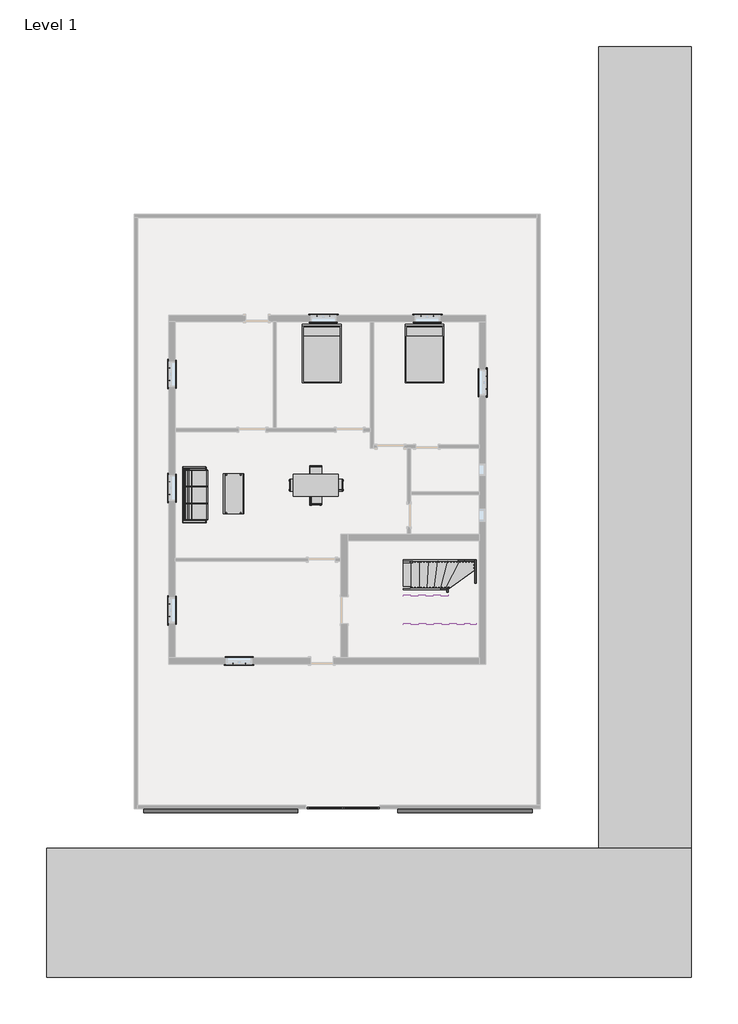
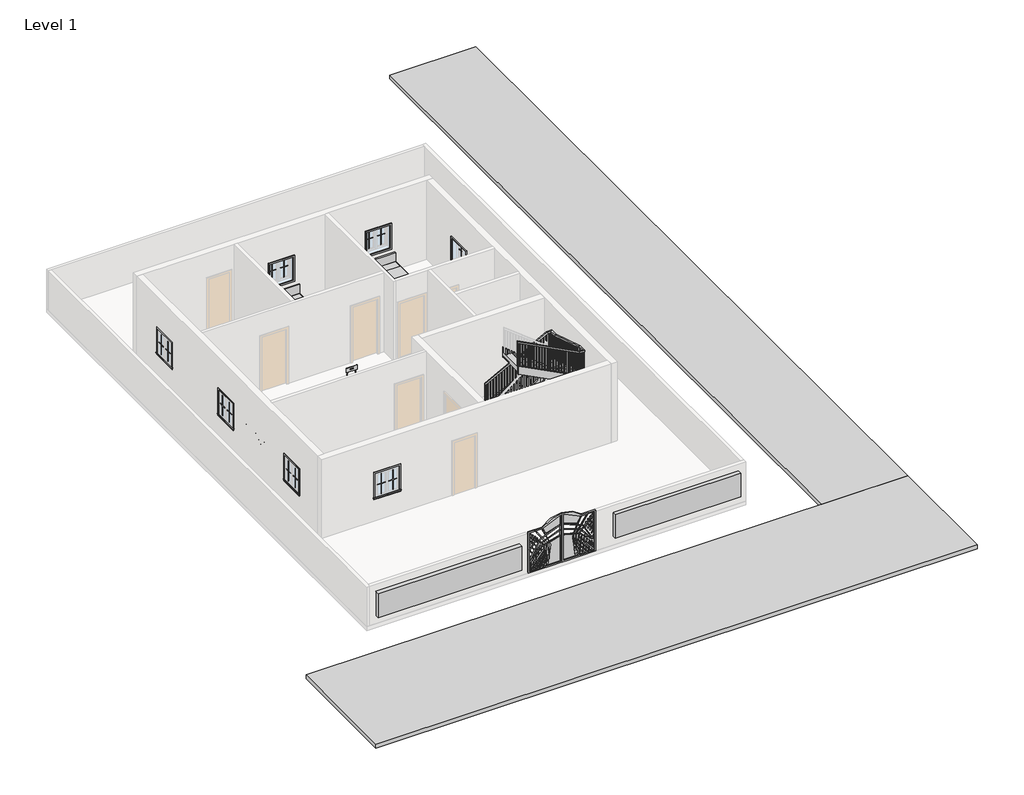
# One storey, part 2 of 2: 33 proxies, 8 members, 4 furniture elements, 1 railing, 1 stair flight.
"""IFC4 building model written with IfcOpenShell, lengths in millimetres."""

from ifc_helpers import new_model, si_unit, frame, origin, place, context, project, spatial, polyline, outline, extrude, faceted_brep, transform, mapped, element, save
from components import generic_models_6bc30956, generic_models_1_generic_models_1_e0ba6133, generic_models_2_generic_models_2_f94be15d, generic_models_3_generic_models_3_0a93b2c0, modern_coffee_table_17989_modern_coffee_table_17989_d3a860c8, muntin_pattern_2x2_muntin_pattern_2x2_b3fe6957, muntin_pattern_2x2_muntin_pattern_2x2_3e0ecaf2, trim_window_exterior_flat_with_sill_41619996, trim_window_interior_flat_picture_frame_51c85655, furniture_2fc85b74, furniture_29a9adb8, furniture_57072a26, bed_17739_bed_17739_15c61121, dining_table_w_chairs_11374_0cdfc61b, stair_flight_a0830a8a

model = new_model("IFC4")

# Units and contexts
model_context = context("Model", 3, world=origin())
ifc_project = project(units=[si_unit("LENGTHUNIT", "METRE", prefix="MILLI")], contexts=[model_context])

# Site, building, storey
site = spatial("IfcSite", under=ifc_project)
building = spatial("IfcBuilding", under=site)
storey = spatial("IfcBuildingStorey", under=building, Name="Level 1", Elevation=0.0)

# Proxies
placement = place(None, origin())
generic_models_shape = generic_models_6bc30956(model_context)
element("IfcBuildingElementProxy", 1, Name="Generic Models", at=placement, inside=storey, context=model_context, shape_type="MappedRepresentation", body=[
    mapped(generic_models_shape, transform((-701.8717864, -9622.1503266, 0.0), x_axis=(1.0, 0.0, 0.0), y_axis=(0.0, 1.0, 0.0), z_axis=(0.0, 0.0, 1.0))),
])
generic_models_1_generic_models_1_shape = generic_models_1_generic_models_1_e0ba6133(model_context)
element("IfcBuildingElementProxy", 2, Name="Generic Models 1 : Generic Models 1", ObjectType="Generic Models 1 : Generic Models 1", at=placement, inside=storey, context=model_context, shape_type="MappedRepresentation", body=[
    mapped(generic_models_1_generic_models_1_shape, transform((0.0, 0.0, 0.0), x_axis=(1.0, 0.0, 0.0), y_axis=(0.0, 1.0, 0.0), z_axis=(0.0, 0.0, 1.0))),
])
generic_models_2_generic_models_2_shape = generic_models_2_generic_models_2_f94be15d(model_context)
element("IfcBuildingElementProxy", 3, Name="Generic Models 2 : Generic Models 2", ObjectType="Generic Models 2 : Generic Models 2", at=placement, inside=storey, context=model_context, shape_type="MappedRepresentation", body=[
    mapped(generic_models_2_generic_models_2_shape, transform((0.0, 0.0, 0.0), x_axis=(1.0, 0.0, 0.0), y_axis=(0.0, 1.0, 0.0), z_axis=(0.0, 0.0, 1.0))),
])
generic_models_3_generic_models_3_shape = generic_models_3_generic_models_3_0a93b2c0(model_context)
element("IfcBuildingElementProxy", 4, Name="Generic Models 3 : Generic Models 3", ObjectType="Generic Models 3 : Generic Models 3", at=placement, inside=storey, context=model_context, shape_type="MappedRepresentation", body=[
    mapped(generic_models_3_generic_models_3_shape, transform((0.0, 0.0, 0.0), x_axis=(1.0, 0.0, 0.0), y_axis=(0.0, 1.0, 0.0), z_axis=(0.0, 0.0, 1.0))),
])
modern_coffee_table_17989_modern_coffee_table_17989_shape = modern_coffee_table_17989_modern_coffee_table_17989_d3a860c8(model_context)
element("IfcBuildingElementProxy", 5, Name="Modern_Coffee_Table_17989 : Modern_Coffee_Table_17989", ObjectType="Modern_Coffee_Table_17989 : Modern_Coffee_Table_17989", at=placement, inside=storey, context=model_context, shape_type="MappedRepresentation", body=[
    mapped(modern_coffee_table_17989_modern_coffee_table_17989_shape, transform((-4791.7841049, 1283.3840961, 0.0), x_axis=(0.0, 1.0, 0.0), y_axis=(-1.0, 0.0, 0.0), z_axis=(0.0, 0.0, 1.0))),
])
muntin_pattern_2x2_muntin_pattern_2x2_shape = muntin_pattern_2x2_muntin_pattern_2x2_b3fe6957(model_context)
element("IfcBuildingElementProxy", 6, Name="Muntin Pattern_2x2 : Muntin Pattern_2x2", ObjectType="Muntin Pattern_2x2 : Muntin Pattern_2x2", at=placement, inside=storey, context=model_context, shape_type="MappedRepresentation", body=[
    mapped(muntin_pattern_2x2_muntin_pattern_2x2_shape, transform((-1586.7442864, 7129.6784997, 984.25), x_axis=(1.0, 0.0, 0.0), y_axis=(0.0, 1.0, 0.0), z_axis=(0.0, 0.0, 1.0))),
])
element("IfcBuildingElementProxy", 7, Name="Muntin Pattern_2x2 : Muntin Pattern_2x2", ObjectType="Muntin Pattern_2x2 : Muntin Pattern_2x2", at=placement, inside=storey, context=model_context, shape_type="MappedRepresentation", body=[
    mapped(muntin_pattern_2x2_muntin_pattern_2x2_shape, transform((1952.1107136, 7129.6784997, 984.25), x_axis=(1.0, 0.0, 0.0), y_axis=(0.0, 1.0, 0.0), z_axis=(0.0, 0.0, 1.0))),
])
element("IfcBuildingElementProxy", 8, Name="Muntin Pattern_2x2 : Muntin Pattern_2x2", ObjectType="Muntin Pattern_2x2 : Muntin Pattern_2x2", at=placement, inside=storey, context=model_context, shape_type="MappedRepresentation", body=[
    mapped(muntin_pattern_2x2_muntin_pattern_2x2_shape, transform((-6633.4067864, 4915.1159997, 984.25), x_axis=(0.0, 1.0, 0.0), y_axis=(-1.0, 0.0, 0.0), z_axis=(0.0, 0.0, 1.0))),
])
element("IfcBuildingElementProxy", 9, Name="Muntin Pattern_2x2 : Muntin Pattern_2x2", ObjectType="Muntin Pattern_2x2 : Muntin Pattern_2x2", at=placement, inside=storey, context=model_context, shape_type="MappedRepresentation", body=[
    mapped(muntin_pattern_2x2_muntin_pattern_2x2_shape, transform((-6633.4067864, 1038.4409997, 984.25), x_axis=(0.0, 1.0, 0.0), y_axis=(-1.0, 0.0, 0.0), z_axis=(0.0, 0.0, 1.0))),
])
element("IfcBuildingElementProxy", 10, Name="Muntin Pattern_2x2 : Muntin Pattern_2x2", ObjectType="Muntin Pattern_2x2 : Muntin Pattern_2x2", at=placement, inside=storey, context=model_context, shape_type="MappedRepresentation", body=[
    mapped(muntin_pattern_2x2_muntin_pattern_2x2_shape, transform((4152.7032136, 5057.9909997, 984.25), x_axis=(0.0, -1.0, 0.0), y_axis=(1.0, 0.0, 0.0), z_axis=(0.0, 0.0, 1.0))),
])
element("IfcBuildingElementProxy", 11, Name="Muntin Pattern_2x2 : Muntin Pattern_2x2", ObjectType="Muntin Pattern_2x2 : Muntin Pattern_2x2", at=placement, inside=storey, context=model_context, shape_type="MappedRepresentation", body=[
    mapped(muntin_pattern_2x2_muntin_pattern_2x2_shape, transform((-6633.4067864, -3125.2540003, 984.25), x_axis=(0.0, 1.0, 0.0), y_axis=(-1.0, 0.0, 0.0), z_axis=(0.0, 0.0, 1.0))),
])
element("IfcBuildingElementProxy", 12, Name="Muntin Pattern_2x2 : Muntin Pattern_2x2", ObjectType="Muntin Pattern_2x2 : Muntin Pattern_2x2", at=placement, inside=storey, context=model_context, shape_type="MappedRepresentation", body=[
    mapped(muntin_pattern_2x2_muntin_pattern_2x2_shape, transform((-4028.3192864, -4738.4715003, 984.25), x_axis=(-1.0, 0.0, 0.0), y_axis=(0.0, -1.0, 0.0), z_axis=(0.0, 0.0, 1.0))),
])
muntin_pattern_2x2_muntin_pattern_2x2_2_shape = muntin_pattern_2x2_muntin_pattern_2x2_3e0ecaf2(model_context)
element("IfcBuildingElementProxy", 13, Name="Muntin Pattern_2x2 : Muntin Pattern_2x2", ObjectType="Muntin Pattern_2x2 : Muntin Pattern_2x2", at=placement, inside=storey, context=model_context, shape_type="MappedRepresentation", body=[
    mapped(muntin_pattern_2x2_muntin_pattern_2x2_2_shape, transform((-1158.1192864, 7129.6784997, 984.25), x_axis=(-1.0, 0.0, 0.0), y_axis=(0.0, -1.0, 0.0), z_axis=(0.0, 0.0, 1.0))),
])
element("IfcBuildingElementProxy", 14, Name="Muntin Pattern_2x2 : Muntin Pattern_2x2", ObjectType="Muntin Pattern_2x2 : Muntin Pattern_2x2", at=placement, inside=storey, context=model_context, shape_type="MappedRepresentation", body=[
    mapped(muntin_pattern_2x2_muntin_pattern_2x2_2_shape, transform((2380.7357136, 7129.6784997, 984.25), x_axis=(-1.0, 0.0, 0.0), y_axis=(0.0, -1.0, 0.0), z_axis=(0.0, 0.0, 1.0))),
])
element("IfcBuildingElementProxy", 15, Name="Muntin Pattern_2x2 : Muntin Pattern_2x2", ObjectType="Muntin Pattern_2x2 : Muntin Pattern_2x2", at=placement, inside=storey, context=model_context, shape_type="MappedRepresentation", body=[
    mapped(muntin_pattern_2x2_muntin_pattern_2x2_2_shape, transform((-6633.4067864, 5343.7409997, 984.25), x_axis=(0.0, -1.0, 0.0), y_axis=(1.0, 0.0, 0.0), z_axis=(0.0, 0.0, 1.0))),
])
element("IfcBuildingElementProxy", 16, Name="Muntin Pattern_2x2 : Muntin Pattern_2x2", ObjectType="Muntin Pattern_2x2 : Muntin Pattern_2x2", at=placement, inside=storey, context=model_context, shape_type="MappedRepresentation", body=[
    mapped(muntin_pattern_2x2_muntin_pattern_2x2_2_shape, transform((-6633.4067864, 1467.0659997, 984.25), x_axis=(0.0, -1.0, 0.0), y_axis=(1.0, 0.0, 0.0), z_axis=(0.0, 0.0, 1.0))),
])
element("IfcBuildingElementProxy", 17, Name="Muntin Pattern_2x2 : Muntin Pattern_2x2", ObjectType="Muntin Pattern_2x2 : Muntin Pattern_2x2", at=placement, inside=storey, context=model_context, shape_type="MappedRepresentation", body=[
    mapped(muntin_pattern_2x2_muntin_pattern_2x2_2_shape, transform((4152.7032136, 4629.3659997, 984.25), x_axis=(0.0, 1.0, 0.0), y_axis=(-1.0, 0.0, 0.0), z_axis=(0.0, 0.0, 1.0))),
])
element("IfcBuildingElementProxy", 18, Name="Muntin Pattern_2x2 : Muntin Pattern_2x2", ObjectType="Muntin Pattern_2x2 : Muntin Pattern_2x2", at=placement, inside=storey, context=model_context, shape_type="MappedRepresentation", body=[
    mapped(muntin_pattern_2x2_muntin_pattern_2x2_2_shape, transform((-6633.4067864, -2696.6290003, 984.25), x_axis=(0.0, -1.0, 0.0), y_axis=(1.0, 0.0, 0.0), z_axis=(0.0, 0.0, 1.0))),
])
element("IfcBuildingElementProxy", 19, Name="Muntin Pattern_2x2 : Muntin Pattern_2x2", ObjectType="Muntin Pattern_2x2 : Muntin Pattern_2x2", at=placement, inside=storey, context=model_context, shape_type="MappedRepresentation", body=[
    mapped(muntin_pattern_2x2_muntin_pattern_2x2_2_shape, transform((-4456.9442864, -4738.4715003, 984.25), x_axis=(1.0, 0.0, 0.0), y_axis=(0.0, 1.0, 0.0), z_axis=(0.0, 0.0, 1.0))),
])
trim_window_exterior_flat_with_sill_shape = trim_window_exterior_flat_with_sill_41619996(model_context)
element("IfcBuildingElementProxy", 20, Name="Trim-Window-Exterior-Flat : with Sill", ObjectType="Trim-Window-Exterior-Flat : with Sill", at=placement, inside=storey, context=model_context, shape_type="MappedRepresentation", body=[
    mapped(trim_window_exterior_flat_with_sill_shape, transform((-1372.4317864, 7139.2034997, 1828.8), x_axis=(-1.0, 0.0, 0.0), y_axis=(0.0, 0.0, 1.0), z_axis=(0.0, 1.0, 0.0))),
])
element("IfcBuildingElementProxy", 21, Name="Trim-Window-Exterior-Flat : with Sill", ObjectType="Trim-Window-Exterior-Flat : with Sill", at=placement, inside=storey, context=model_context, shape_type="MappedRepresentation", body=[
    mapped(trim_window_exterior_flat_with_sill_shape, transform((2166.4232136, 7139.2034997, 1828.8), x_axis=(-1.0, 0.0, 0.0), y_axis=(0.0, 0.0, 1.0), z_axis=(0.0, 1.0, 0.0))),
])
element("IfcBuildingElementProxy", 22, Name="Trim-Window-Exterior-Flat : with Sill", ObjectType="Trim-Window-Exterior-Flat : with Sill", at=placement, inside=storey, context=model_context, shape_type="MappedRepresentation", body=[
    mapped(trim_window_exterior_flat_with_sill_shape, transform((-6642.9317864, 5129.4284997, 1828.8), x_axis=(0.0, -1.0, 0.0), y_axis=(0.0, 0.0, 1.0), z_axis=(-1.0, 0.0, 0.0))),
])
element("IfcBuildingElementProxy", 23, Name="Trim-Window-Exterior-Flat : with Sill", ObjectType="Trim-Window-Exterior-Flat : with Sill", at=placement, inside=storey, context=model_context, shape_type="MappedRepresentation", body=[
    mapped(trim_window_exterior_flat_with_sill_shape, transform((-6642.9317864, 1252.7534997, 1828.8), x_axis=(0.0, -1.0, 0.0), y_axis=(0.0, 0.0, 1.0), z_axis=(-1.0, 0.0, 0.0))),
])
element("IfcBuildingElementProxy", 24, Name="Trim-Window-Exterior-Flat : with Sill", ObjectType="Trim-Window-Exterior-Flat : with Sill", at=placement, inside=storey, context=model_context, shape_type="MappedRepresentation", body=[
    mapped(trim_window_exterior_flat_with_sill_shape, transform((4162.2282136, 4843.6784997, 1828.8), x_axis=(0.0, 1.0, 0.0), y_axis=(0.0, 0.0, 1.0), z_axis=(1.0, 0.0, 0.0))),
])
element("IfcBuildingElementProxy", 25, Name="Trim-Window-Exterior-Flat : with Sill", ObjectType="Trim-Window-Exterior-Flat : with Sill", at=placement, inside=storey, context=model_context, shape_type="MappedRepresentation", body=[
    mapped(trim_window_exterior_flat_with_sill_shape, transform((-6642.9317864, -2910.9415003, 1828.8), x_axis=(0.0, -1.0, 0.0), y_axis=(0.0, 0.0, 1.0), z_axis=(-1.0, 0.0, 0.0))),
])
element("IfcBuildingElementProxy", 26, Name="Trim-Window-Exterior-Flat : with Sill", ObjectType="Trim-Window-Exterior-Flat : with Sill", at=placement, inside=storey, context=model_context, shape_type="MappedRepresentation", body=[
    mapped(trim_window_exterior_flat_with_sill_shape, transform((-4242.6317864, -4747.9965003, 1828.8), x_axis=(1.0, 0.0, 0.0), y_axis=(0.0, 0.0, 1.0), z_axis=(0.0, -1.0, 0.0))),
])
trim_window_interior_flat_picture_frame_shape = trim_window_interior_flat_picture_frame_51c85655(model_context)
element("IfcBuildingElementProxy", 27, Name="Trim-Window-Interior-Flat : Picture Frame", ObjectType="Trim-Window-Interior-Flat : Picture Frame", at=placement, inside=storey, context=model_context, shape_type="MappedRepresentation", body=[
    mapped(trim_window_interior_flat_picture_frame_shape, transform((-1372.4317864, 6910.6034997, 1828.8), x_axis=(1.0, 0.0, 0.0), y_axis=(0.0, 0.0, 1.0), z_axis=(0.0, -1.0, 0.0))),
])
element("IfcBuildingElementProxy", 28, Name="Trim-Window-Interior-Flat : Picture Frame", ObjectType="Trim-Window-Interior-Flat : Picture Frame", at=placement, inside=storey, context=model_context, shape_type="MappedRepresentation", body=[
    mapped(trim_window_interior_flat_picture_frame_shape, transform((2166.4232136, 6910.6034997, 1828.8), x_axis=(1.0, 0.0, 0.0), y_axis=(0.0, 0.0, 1.0), z_axis=(0.0, -1.0, 0.0))),
])
element("IfcBuildingElementProxy", 29, Name="Trim-Window-Interior-Flat : Picture Frame", ObjectType="Trim-Window-Interior-Flat : Picture Frame", at=placement, inside=storey, context=model_context, shape_type="MappedRepresentation", body=[
    mapped(trim_window_interior_flat_picture_frame_shape, transform((-6414.3317864, 5129.4284997, 1828.8), x_axis=(0.0, 1.0, 0.0), y_axis=(0.0, 0.0, 1.0), z_axis=(1.0, 0.0, 0.0))),
])
element("IfcBuildingElementProxy", 30, Name="Trim-Window-Interior-Flat : Picture Frame", ObjectType="Trim-Window-Interior-Flat : Picture Frame", at=placement, inside=storey, context=model_context, shape_type="MappedRepresentation", body=[
    mapped(trim_window_interior_flat_picture_frame_shape, transform((-6414.3317864, 1252.7534997, 1828.8), x_axis=(0.0, 1.0, 0.0), y_axis=(0.0, 0.0, 1.0), z_axis=(1.0, 0.0, 0.0))),
])
element("IfcBuildingElementProxy", 31, Name="Trim-Window-Interior-Flat : Picture Frame", ObjectType="Trim-Window-Interior-Flat : Picture Frame", at=placement, inside=storey, context=model_context, shape_type="MappedRepresentation", body=[
    mapped(trim_window_interior_flat_picture_frame_shape, transform((3933.6282136, 4843.6784997, 1828.8), x_axis=(0.0, -1.0, 0.0), y_axis=(0.0, 0.0, 1.0), z_axis=(-1.0, 0.0, 0.0))),
])
element("IfcBuildingElementProxy", 32, Name="Trim-Window-Interior-Flat : Picture Frame", ObjectType="Trim-Window-Interior-Flat : Picture Frame", at=placement, inside=storey, context=model_context, shape_type="MappedRepresentation", body=[
    mapped(trim_window_interior_flat_picture_frame_shape, transform((-6414.3317864, -2910.9415003, 1828.8), x_axis=(0.0, 1.0, 0.0), y_axis=(0.0, 0.0, 1.0), z_axis=(1.0, 0.0, 0.0))),
])
element("IfcBuildingElementProxy", 33, Name="Trim-Window-Interior-Flat : Picture Frame", ObjectType="Trim-Window-Interior-Flat : Picture Frame", at=placement, inside=storey, context=model_context, shape_type="MappedRepresentation", body=[
    mapped(trim_window_interior_flat_picture_frame_shape, transform((-4242.6317864, -4519.3965003, 1828.8), x_axis=(-1.0, 0.0, 0.0), y_axis=(0.0, 0.0, 1.0), z_axis=(0.0, 1.0, 0.0))),
])

# Furniture
furniture_shape = furniture_2fc85b74(model_context)
furniture_2_shape = furniture_29a9adb8(model_context)
furniture_3_shape = furniture_57072a26(model_context)
element("IfcFurniture", 34, at=placement, inside=storey, context=model_context, shape_type="MappedRepresentation", body=[
    mapped(furniture_shape, transform((-5371.0104604, 1017.8034997, 0.0), x_axis=(0.0, 1.0, 0.0), y_axis=(-1.0, 0.0, 0.0), z_axis=(0.0, 0.0, 1.0))),
    mapped(furniture_2_shape, transform((-5371.0104604, 1017.8034997, 0.0), x_axis=(0.0, 1.0, 0.0), y_axis=(-1.0, 0.0, 0.0), z_axis=(0.0, 0.0, 1.0))),
    mapped(furniture_3_shape, transform((-5371.0104604, 1017.8034997, 0.0), x_axis=(0.0, 1.0, 0.0), y_axis=(-1.0, 0.0, 0.0), z_axis=(0.0, 0.0, 1.0))),
])
bed_17739_bed_17739_shape = bed_17739_bed_17739_15c61121(model_context)
element("IfcFurniture", 35, ObjectType="Bed_17739 : Bed_17739", at=placement, inside=storey, context=model_context, shape_type="MappedRepresentation", body=[
    mapped(bed_17739_bed_17739_shape, transform((-1425.7717864, 5805.7034997, 0.0), x_axis=(1.0, 0.0, 0.0), y_axis=(0.0, 1.0, 0.0), z_axis=(0.0, 0.0, 1.0))),
])
element("IfcFurniture", 36, ObjectType="Bed_17739 : Bed_17739", at=placement, inside=storey, context=model_context, shape_type="MappedRepresentation", body=[
    mapped(bed_17739_bed_17739_shape, transform((2066.7282136, 5805.7034997, 0.0), x_axis=(1.0, 0.0, 0.0), y_axis=(0.0, 1.0, 0.0), z_axis=(0.0, 0.0, 1.0))),
])
dining_table_w_chairs_11374_shape = dining_table_w_chairs_11374_0cdfc61b(model_context)
element("IfcFurniture", 37, ObjectType="Dining_Table_w_Chairs_11374", at=placement, inside=storey, context=model_context, shape_type="MappedRepresentation", body=[
    mapped(dining_table_w_chairs_11374_shape, transform((-1657.0397106, 1252.0888157, 0.0), x_axis=(1.0, 0.0, 0.0), y_axis=(0.0, 1.0, 0.0), z_axis=(0.0, 0.0, 1.0))),
])

# Members
element("IfcMember", 38, ObjectType="Stringer - 2\" Width", at=placement, inside=storey, context=model_context, shape_type="SweptSolid", body=[
    extrude(outline(polyline([(229.639954, 1342.8282136), (0.0, 1342.8282136), (0.0, 1562.5905312), (962.500629, 3430.2454053), (1305.3956453, 3430.2454053), (229.639954, 1342.8282136)])), frame((0.0, -1245.3365003, 0.0), z_axis=(0.0, 1.0, 0.0), x_axis=(0.0, 0.0, 1.0)), (0.0, 0.0, 1.0), 50.8),
])
element("IfcMember", 39, ObjectType="Stringer - 2\" Width", at=placement, inside=storey, context=model_context, shape_type="SweptSolid", body=[
    extrude(outline(polyline([(3430.2454053, -1245.3365003), (3430.2454053, -1194.5365003), (3784.9599055, -1194.5365003), (3784.9599055, -1245.3365003), (3430.2454053, -1245.3365003)])), frame((0.0, 0.0, 962.500629), z_axis=(0.0, 0.0, 1.0), x_axis=(1.0, 0.0, 0.0)), (0.0, 0.0, 1.0), 342.8950162),
])
element("IfcMember", 40, ObjectType="Stringer - 2\" Width", at=placement, inside=storey, context=model_context, shape_type="SweptSolid", body=[
    extrude(outline(polyline([(-1194.5365003, 1289.0952212), (-1194.5365003, 1000.5956453), (-1364.0589833, 1000.5956453), (-3353.5365003, 1638.9682298), (-3353.5365003, 1969.9972697), (-3316.5563831, 1969.9972697), (-1194.5365003, 1289.0952212)])), frame((3784.9599055, 0.0, 0.0), z_axis=(1.0, 0.0, 0.0), x_axis=(0.0, 1.0, 0.0)), (0.0, 0.0, 1.0), 50.8),
])
element("IfcMember", 41, ObjectType="Stringer - 2\" Width", at=placement, inside=storey, context=model_context, shape_type="SweptSolid", body=[
    extrude(outline(polyline([(3835.7599055, -3353.5365003), (3835.7599055, -3404.3365003), (3430.2454053, -3404.3365003), (3430.2454053, -3353.5365003), (3835.7599055, -3353.5365003)])), frame((0.0, 0.0, 1649.8904473), z_axis=(0.0, 0.0, 1.0), x_axis=(1.0, 0.0, 0.0)), (0.0, 0.0, 1.0), 320.1068224),
])
element("IfcMember", 42, ObjectType="Stringer - 2\" Width", at=placement, inside=storey, context=model_context, shape_type="SweptSolid", body=[
    extrude(outline(polyline([(1649.8904473, 3430.2454053), (1969.9972697, 3430.2454053), (3045.7529609, 1342.8282136), (2725.6461385, 1342.8282136), (1649.8904473, 3430.2454053)])), frame((0.0, -3404.3365003, 0.0), z_axis=(0.0, 1.0, 0.0), x_axis=(0.0, 0.0, 1.0)), (0.0, 0.0, 1.0), 50.8),
])
element("IfcMember", 43, ObjectType="Stringer - 2\" Width", at=placement, inside=storey, context=model_context, shape_type="SweptSolid", body=[
    extrude(outline(polyline([(176.1764461, 1342.8282136), (0.0, 1342.8282136), (0.0, 1609.0898582), (987.1410923, 2819.7599055), (1380.418648, 2819.7599055), (176.1764461, 1342.8282136)])), frame((0.0, -2210.5365003, 0.0), z_axis=(0.0, 1.0, 0.0), x_axis=(0.0, 0.0, 1.0)), (0.0, 0.0, 1.0), 50.8),
])
element("IfcMember", 44, ObjectType="Stringer - 2\" Width", at=placement, inside=storey, context=model_context, shape_type="SweptSolid", body=[
    extrude(outline(polyline([(-2159.7365003, 1573.2682978), (-2159.7365003, 1028.5617647), (-2193.9787177, 1028.5617647), (-2388.3365003, 1360.465107), (-2388.3365003, 1926.1409689), (-2366.3736178, 1926.1409689), (-2159.7365003, 1573.2682978)])), frame((2819.7599055, 0.0, 0.0), z_axis=(1.0, 0.0, 0.0), x_axis=(0.0, 1.0, 0.0)), (0.0, 0.0, 1.0), 50.8),
])
element("IfcMember", 45, ObjectType="Stringer - 2\" Width", at=placement, inside=storey, context=model_context, shape_type="SweptSolid", body=[
    extrude(outline(polyline([(1532.8634131, 2870.5599055), (1926.1409689, 2870.5599055), (3171.8038432, 1342.8282136), (2778.5262875, 1342.8282136), (1532.8634131, 2870.5599055)])), frame((0.0, -2439.1365003, 0.0), z_axis=(0.0, 1.0, 0.0), x_axis=(0.0, 0.0, 1.0)), (0.0, 0.0, 1.0), 50.8),
])

# Railing
element("IfcRailing", 46, ObjectType="Handrail - Rectangular", at=placement, inside=storey, context=model_context, shape_type="SolidModel", body=[
    faceted_brep([(1342.8282136, -1245.3365003, 1083.7333333), (1342.8282136, -1245.3365003, 1026.2742652), (1342.8282136, -1296.1365003, 1026.2742652), (1342.8282136, -1296.1365003, 1083.7333333), (3600.5532757, -1245.3365003, 2277.0239201), (3613.1523402, -1245.3365003, 2226.2239201), (3613.1523402, -1296.1365003, 2226.2239201), (3600.5532757, -1296.1365003, 2277.0239201), (3784.9599055, -1245.3365003, 2277.0239201), (3784.9599055, -1245.3365003, 2226.2239201), (3734.1599055, -1296.1365003, 2226.2239201), (3734.1599055, -1296.1365003, 2277.0239201), (3784.9599055, -1532.6483825, 2277.0239201), (3784.9599055, -1540.5989586, 2226.2239201), (3734.1599055, -1540.5989586, 2226.2239201), (3734.1599055, -1532.6483825, 2277.0239201), (3784.9599055, -3066.2246182, 2769.1094132), (3784.9599055, -3074.1751943, 2718.3094132), (3734.1599055, -3074.1751943, 2718.3094132), (3734.1599055, -3066.2246182, 2769.1094132), (3784.9599055, -3353.5365003, 2769.1094132), (3784.9599055, -3353.5365003, 2718.3094132), (3734.1599055, -3302.7365003, 2718.3094132), (3734.1599055, -3302.7365003, 2769.1094132), (3600.5532757, -3353.5365003, 2769.1094132), (3587.9542112, -3353.5365003, 2718.3094132), (3587.9542112, -3302.7365003, 2718.3094132), (3600.5532757, -3302.7365003, 2769.1094132), (1342.8282136, -3353.5365003, 3962.4), (1342.8282136, -3302.7365003, 3962.4), (1342.8282136, -3302.7365003, 3904.9409318), (1342.8282136, -3353.5365003, 3904.9409318)], [[[0, 1, 2, 3]], [[1, 0, 4, 5]], [[2, 1, 5, 6]], [[3, 2, 6, 7]], [[0, 3, 7, 4]], [[5, 4, 8, 9]], [[6, 5, 9, 10]], [[7, 6, 10, 11]], [[4, 7, 11, 8]], [[9, 8, 12, 13]], [[10, 9, 13, 14]], [[11, 10, 14, 15]], [[8, 11, 15, 12]], [[13, 12, 16, 17]], [[14, 13, 17, 18]], [[15, 14, 18, 19]], [[12, 15, 19, 16]], [[17, 16, 20, 21]], [[18, 17, 21, 22]], [[19, 18, 22, 23]], [[16, 19, 23, 20]], [[21, 20, 24, 25]], [[22, 21, 25, 26]], [[23, 22, 26, 27]], [[20, 23, 27, 24]], [[28, 29, 30, 31]], [[25, 24, 28, 31]], [[26, 25, 31, 30]], [[27, 26, 30, 29]], [[24, 27, 29, 28]]]),
    extrude(outline(polyline([(3867.7284102, 1413.2349055), (2878.6666667, 1413.2349055), (2878.6666667, 1432.2849055), (3857.6597858, 1432.2849055), (3867.7284102, 1413.2349055)])), frame((0.0, -3337.6615003, 0.0), z_axis=(0.0, 1.0, 0.0), x_axis=(0.0, 0.0, 1.0)), (0.0, 0.0, 1.0), 19.05),
    extrude(outline(polyline([(3814.02908, 1514.8349055), (2878.6666667, 1514.8349055), (2878.6666667, 1533.8849055), (3803.9604556, 1533.8849055), (3814.02908, 1514.8349055)])), frame((0.0, -3337.6615003, 0.0), z_axis=(0.0, 1.0, 0.0), x_axis=(0.0, 0.0, 1.0)), (0.0, 0.0, 1.0), 19.05),
    extrude(outline(polyline([(3760.3297498, 1616.4349055), (2709.3333333, 1616.4349055), (2709.3333333, 1635.4849055), (3750.2611254, 1635.4849055), (3760.3297498, 1616.4349055)])), frame((0.0, -3337.6615003, 0.0), z_axis=(0.0, 1.0, 0.0), x_axis=(0.0, 0.0, 1.0)), (0.0, 0.0, 1.0), 19.05),
    extrude(outline(polyline([(3706.6304196, 1718.0349055), (2709.3333333, 1718.0349055), (2709.3333333, 1737.0849055), (3696.5617952, 1737.0849055), (3706.6304196, 1718.0349055)])), frame((0.0, -3337.6615003, 0.0), z_axis=(0.0, 1.0, 0.0), x_axis=(0.0, 0.0, 1.0)), (0.0, 0.0, 1.0), 19.05),
    extrude(outline(polyline([(3652.9310894, 1819.6349055), (2709.3333333, 1819.6349055), (2709.3333333, 1838.6849055), (3642.862465, 1838.6849055), (3652.9310894, 1819.6349055)])), frame((0.0, -3337.6615003, 0.0), z_axis=(0.0, 1.0, 0.0), x_axis=(0.0, 0.0, 1.0)), (0.0, 0.0, 1.0), 19.05),
    extrude(outline(polyline([(3599.2317592, 1921.2349055), (2540.0, 1921.2349055), (2540.0, 1940.2849055), (3589.1631348, 1940.2849055), (3599.2317592, 1921.2349055)])), frame((0.0, -3337.6615003, 0.0), z_axis=(0.0, 1.0, 0.0), x_axis=(0.0, 0.0, 1.0)), (0.0, 0.0, 1.0), 19.05),
    extrude(outline(polyline([(3545.532429, 2022.8349055), (2540.0, 2022.8349055), (2540.0, 2041.8849055), (3535.4638046, 2041.8849055), (3545.532429, 2022.8349055)])), frame((0.0, -3337.6615003, 0.0), z_axis=(0.0, 1.0, 0.0), x_axis=(0.0, 0.0, 1.0)), (0.0, 0.0, 1.0), 19.05),
    extrude(outline(polyline([(3491.8330988, 2124.4349055), (2540.0, 2124.4349055), (2540.0, 2143.4849055), (3481.7644744, 2143.4849055), (3491.8330988, 2124.4349055)])), frame((0.0, -3337.6615003, 0.0), z_axis=(0.0, 1.0, 0.0), x_axis=(0.0, 0.0, 1.0)), (0.0, 0.0, 1.0), 19.05),
    extrude(outline(polyline([(3438.1337686, 2226.0349055), (2370.6666667, 2226.0349055), (2370.6666667, 2245.0849055), (3428.0651442, 2245.0849055), (3438.1337686, 2226.0349055)])), frame((0.0, -3337.6615003, 0.0), z_axis=(0.0, 1.0, 0.0), x_axis=(0.0, 0.0, 1.0)), (0.0, 0.0, 1.0), 19.05),
    extrude(outline(polyline([(3384.4344384, 2327.6349055), (2370.6666667, 2327.6349055), (2370.6666667, 2346.6849055), (3374.365814, 2346.6849055), (3384.4344384, 2327.6349055)])), frame((0.0, -3337.6615003, 0.0), z_axis=(0.0, 1.0, 0.0), x_axis=(0.0, 0.0, 1.0)), (0.0, 0.0, 1.0), 19.05),
    extrude(outline(polyline([(3330.7351082, 2429.2349055), (2370.6666667, 2429.2349055), (2370.6666667, 2448.2849055), (3320.6664838, 2448.2849055), (3330.7351082, 2429.2349055)])), frame((0.0, -3337.6615003, 0.0), z_axis=(0.0, 1.0, 0.0), x_axis=(0.0, 0.0, 1.0)), (0.0, 0.0, 1.0), 19.05),
    extrude(outline(polyline([(3277.035778, 2530.8349055), (2201.3333333, 2530.8349055), (2201.3333333, 2549.8849055), (3266.9671536, 2549.8849055), (3277.035778, 2530.8349055)])), frame((0.0, -3337.6615003, 0.0), z_axis=(0.0, 1.0, 0.0), x_axis=(0.0, 0.0, 1.0)), (0.0, 0.0, 1.0), 19.05),
    extrude(outline(polyline([(3223.3364478, 2632.4349055), (2201.3333333, 2632.4349055), (2201.3333333, 2651.4849055), (3213.2678234, 2651.4849055), (3223.3364478, 2632.4349055)])), frame((0.0, -3337.6615003, 0.0), z_axis=(0.0, 1.0, 0.0), x_axis=(0.0, 0.0, 1.0)), (0.0, 0.0, 1.0), 19.05),
    extrude(outline(polyline([(3169.6371176, 2734.0349055), (2201.3333333, 2734.0349055), (2201.3333333, 2753.0849055), (3159.5684932, 2753.0849055), (3169.6371176, 2734.0349055)])), frame((0.0, -3337.6615003, 0.0), z_axis=(0.0, 1.0, 0.0), x_axis=(0.0, 0.0, 1.0)), (0.0, 0.0, 1.0), 19.05),
    extrude(outline(polyline([(3115.9377874, 2835.6349055), (2201.3333333, 2835.6349055), (2201.3333333, 2854.6849055), (3105.869163, 2854.6849055), (3115.9377874, 2835.6349055)])), frame((0.0, -3337.6615003, 0.0), z_axis=(0.0, 1.0, 0.0), x_axis=(0.0, 0.0, 1.0)), (0.0, 0.0, 1.0), 19.05),
    extrude(outline(polyline([(3062.2384572, 2937.2349055), (2032.0, 2937.2349055), (2032.0, 2956.2849055), (3052.1698328, 2956.2849055), (3062.2384572, 2937.2349055)])), frame((0.0, -3337.6615003, 0.0), z_axis=(0.0, 1.0, 0.0), x_axis=(0.0, 0.0, 1.0)), (0.0, 0.0, 1.0), 19.05),
    extrude(outline(polyline([(3008.539127, 3038.8349055), (2032.0, 3038.8349055), (2032.0, 3057.8849055), (2998.4705026, 3057.8849055), (3008.539127, 3038.8349055)])), frame((0.0, -3337.6615003, 0.0), z_axis=(0.0, 1.0, 0.0), x_axis=(0.0, 0.0, 1.0)), (0.0, 0.0, 1.0), 19.05),
    extrude(outline(polyline([(2954.8397968, 3140.4349055), (2032.0, 3140.4349055), (2032.0, 3159.4849055), (2944.7711724, 3159.4849055), (2954.8397968, 3140.4349055)])), frame((0.0, -3337.6615003, 0.0), z_axis=(0.0, 1.0, 0.0), x_axis=(0.0, 0.0, 1.0)), (0.0, 0.0, 1.0), 19.05),
    extrude(outline(polyline([(2901.1404666, 3242.0349055), (2032.0, 3242.0349055), (2032.0, 3261.0849055), (2891.0718422, 3261.0849055), (2901.1404666, 3242.0349055)])), frame((0.0, -3337.6615003, 0.0), z_axis=(0.0, 1.0, 0.0), x_axis=(0.0, 0.0, 1.0)), (0.0, 0.0, 1.0), 19.05),
    extrude(outline(polyline([(2847.4411364, 3343.6349055), (1862.6666667, 3343.6349055), (1862.6666667, 3362.6849055), (2837.372512, 3362.6849055), (2847.4411364, 3343.6349055)])), frame((0.0, -3337.6615003, 0.0), z_axis=(0.0, 1.0, 0.0), x_axis=(0.0, 0.0, 1.0)), (0.0, 0.0, 1.0), 19.05),
    extrude(outline(polyline([(2793.7418062, 3445.2349055), (1862.6666667, 3445.2349055), (1862.6666667, 3464.2849055), (2783.6731818, 3464.2849055), (2793.7418062, 3445.2349055)])), frame((0.0, -3337.6615003, 0.0), z_axis=(0.0, 1.0, 0.0), x_axis=(0.0, 0.0, 1.0)), (0.0, 0.0, 1.0), 19.05),
    extrude(outline(polyline([(2740.042476, 3546.8349055), (1862.6666667, 3546.8349055), (1862.6666667, 3565.8849055), (2729.9738516, 3565.8849055), (2740.042476, 3546.8349055)])), frame((0.0, -3337.6615003, 0.0), z_axis=(0.0, 1.0, 0.0), x_axis=(0.0, 0.0, 1.0)), (0.0, 0.0, 1.0), 19.05),
    extrude(outline(polyline([(3667.4849055, -3337.6615003), (3648.4349055, -3337.6615003), (3648.4349055, -3318.6115003), (3667.4849055, -3318.6115003), (3667.4849055, -3337.6615003)])), frame((0.0, 0.0, 1862.6666667), z_axis=(0.0, 0.0, 1.0), x_axis=(1.0, 0.0, 0.0)), (0.0, 0.0, 1.0), 855.6427466),
    extrude(outline(polyline([(3769.0849055, -3293.2115003), (3769.0849055, -3312.2615003), (3750.0349055, -3312.2615003), (3750.0349055, -3293.2115003), (3769.0849055, -3293.2115003)])), frame((0.0, 0.0, 1862.6666667), z_axis=(0.0, 0.0, 1.0), x_axis=(1.0, 0.0, 0.0)), (0.0, 0.0, 1.0), 855.6427466),
    extrude(outline(polyline([(3769.0849055, -3191.6115003), (3769.0849055, -3210.6615003), (3750.0349055, -3210.6615003), (3750.0349055, -3191.6115003), (3769.0849055, -3191.6115003)])), frame((0.0, 0.0, 1862.6666667), z_axis=(0.0, 0.0, 1.0), x_axis=(1.0, 0.0, 0.0)), (0.0, 0.0, 1.0), 855.6427466),
    extrude(outline(polyline([(3769.0849055, -3090.0115003), (3769.0849055, -3109.0615003), (3750.0349055, -3109.0615003), (3750.0349055, -3090.0115003), (3769.0849055, -3090.0115003)])), frame((0.0, 0.0, 1862.6666667), z_axis=(0.0, 0.0, 1.0), x_axis=(1.0, 0.0, 0.0)), (0.0, 0.0, 1.0), 855.6427466),
    extrude(outline(polyline([(-2988.4115003, 2690.7900316), (-2988.4115003, 1693.3333333), (-3007.4615003, 1693.3333333), (-3007.4615003, 2696.9026907), (-2988.4115003, 2690.7900316)])), frame((3750.0349055, 0.0, 0.0), z_axis=(1.0, 0.0, 0.0), x_axis=(0.0, 1.0, 0.0)), (0.0, 0.0, 1.0), 19.05),
    extrude(outline(polyline([(-2886.8115003, 2658.1891834), (-2886.8115003, 1693.3333333), (-2905.8615003, 1693.3333333), (-2905.8615003, 2664.3018425), (-2886.8115003, 2658.1891834)])), frame((3750.0349055, 0.0, 0.0), z_axis=(1.0, 0.0, 0.0), x_axis=(0.0, 1.0, 0.0)), (0.0, 0.0, 1.0), 19.05),
    extrude(outline(polyline([(-2785.2115003, 2625.5883352), (-2785.2115003, 1693.3333333), (-2804.2615003, 1693.3333333), (-2804.2615003, 2631.7009942), (-2785.2115003, 2625.5883352)])), frame((3750.0349055, 0.0, 0.0), z_axis=(1.0, 0.0, 0.0), x_axis=(0.0, 1.0, 0.0)), (0.0, 0.0, 1.0), 19.05),
    extrude(outline(polyline([(-2683.6115003, 2592.987487), (-2683.6115003, 1693.3333333), (-2702.6615003, 1693.3333333), (-2702.6615003, 2599.100146), (-2683.6115003, 2592.987487)])), frame((3750.0349055, 0.0, 0.0), z_axis=(1.0, 0.0, 0.0), x_axis=(0.0, 1.0, 0.0)), (0.0, 0.0, 1.0), 19.05),
    extrude(outline(polyline([(-2582.0115003, 2560.3866387), (-2582.0115003, 1693.3333333), (-2601.0615003, 1693.3333333), (-2601.0615003, 2566.4992978), (-2582.0115003, 2560.3866387)])), frame((3750.0349055, 0.0, 0.0), z_axis=(1.0, 0.0, 0.0), x_axis=(0.0, 1.0, 0.0)), (0.0, 0.0, 1.0), 19.05),
    extrude(outline(polyline([(-2480.4115003, 2527.7857905), (-2480.4115003, 1524.0), (-2499.4615003, 1524.0), (-2499.4615003, 2533.8984495), (-2480.4115003, 2527.7857905)])), frame((3750.0349055, 0.0, 0.0), z_axis=(1.0, 0.0, 0.0), x_axis=(0.0, 1.0, 0.0)), (0.0, 0.0, 1.0), 19.05),
    extrude(outline(polyline([(-2378.8115003, 2495.1849423), (-2378.8115003, 1524.0), (-2397.8615003, 1524.0), (-2397.8615003, 2501.2976013), (-2378.8115003, 2495.1849423)])), frame((3750.0349055, 0.0, 0.0), z_axis=(1.0, 0.0, 0.0), x_axis=(0.0, 1.0, 0.0)), (0.0, 0.0, 1.0), 19.05),
    extrude(outline(polyline([(-2277.2115003, 2462.5840941), (-2277.2115003, 1524.0), (-2296.2615003, 1524.0), (-2296.2615003, 2468.6967531), (-2277.2115003, 2462.5840941)])), frame((3750.0349055, 0.0, 0.0), z_axis=(1.0, 0.0, 0.0), x_axis=(0.0, 1.0, 0.0)), (0.0, 0.0, 1.0), 19.05),
    extrude(outline(polyline([(-2175.6115003, 2429.9832458), (-2175.6115003, 1524.0), (-2194.6615003, 1524.0), (-2194.6615003, 2436.0959049), (-2175.6115003, 2429.9832458)])), frame((3750.0349055, 0.0, 0.0), z_axis=(1.0, 0.0, 0.0), x_axis=(0.0, 1.0, 0.0)), (0.0, 0.0, 1.0), 19.05),
    extrude(outline(polyline([(-2074.0115003, 2397.3823976), (-2074.0115003, 1524.0), (-2093.0615003, 1524.0), (-2093.0615003, 2403.4950566), (-2074.0115003, 2397.3823976)])), frame((3750.0349055, 0.0, 0.0), z_axis=(1.0, 0.0, 0.0), x_axis=(0.0, 1.0, 0.0)), (0.0, 0.0, 1.0), 19.05),
    extrude(outline(polyline([(-1972.4115003, 2364.7815494), (-1972.4115003, 1354.6666667), (-1991.4615003, 1354.6666667), (-1991.4615003, 2370.8942084), (-1972.4115003, 2364.7815494)])), frame((3750.0349055, 0.0, 0.0), z_axis=(1.0, 0.0, 0.0), x_axis=(0.0, 1.0, 0.0)), (0.0, 0.0, 1.0), 19.05),
    extrude(outline(polyline([(-1870.8115003, 2332.1807011), (-1870.8115003, 1354.6666667), (-1889.8615003, 1354.6666667), (-1889.8615003, 2338.2933602), (-1870.8115003, 2332.1807011)])), frame((3750.0349055, 0.0, 0.0), z_axis=(1.0, 0.0, 0.0), x_axis=(0.0, 1.0, 0.0)), (0.0, 0.0, 1.0), 19.05),
    extrude(outline(polyline([(-1769.2115003, 2299.5798529), (-1769.2115003, 1354.6666667), (-1788.2615003, 1354.6666667), (-1788.2615003, 2305.692512), (-1769.2115003, 2299.5798529)])), frame((3750.0349055, 0.0, 0.0), z_axis=(1.0, 0.0, 0.0), x_axis=(0.0, 1.0, 0.0)), (0.0, 0.0, 1.0), 19.05),
    extrude(outline(polyline([(-1667.6115003, 2266.9790047), (-1667.6115003, 1354.6666667), (-1686.6615003, 1354.6666667), (-1686.6615003, 2273.0916637), (-1667.6115003, 2266.9790047)])), frame((3750.0349055, 0.0, 0.0), z_axis=(1.0, 0.0, 0.0), x_axis=(0.0, 1.0, 0.0)), (0.0, 0.0, 1.0), 19.05),
    extrude(outline(polyline([(-1566.0115003, 2234.3781565), (-1566.0115003, 1354.6666667), (-1585.0615003, 1354.6666667), (-1585.0615003, 2240.4908155), (-1566.0115003, 2234.3781565)])), frame((3750.0349055, 0.0, 0.0), z_axis=(1.0, 0.0, 0.0), x_axis=(0.0, 1.0, 0.0)), (0.0, 0.0, 1.0), 19.05),
    extrude(outline(polyline([(3769.0849055, -1464.4115003), (3769.0849055, -1483.4615003), (3750.0349055, -1483.4615003), (3750.0349055, -1464.4115003), (3769.0849055, -1464.4115003)])), frame((0.0, 0.0, 1185.3333333), z_axis=(0.0, 0.0, 1.0), x_axis=(1.0, 0.0, 0.0)), (0.0, 0.0, 1.0), 1040.8905868),
    extrude(outline(polyline([(3769.0849055, -1362.8115003), (3769.0849055, -1381.8615003), (3750.0349055, -1381.8615003), (3750.0349055, -1362.8115003), (3769.0849055, -1362.8115003)])), frame((0.0, 0.0, 1185.3333333), z_axis=(0.0, 0.0, 1.0), x_axis=(1.0, 0.0, 0.0)), (0.0, 0.0, 1.0), 1040.8905868),
    extrude(outline(polyline([(3670.1032136, -1261.2115003), (3689.1532136, -1261.2115003), (3689.1532136, -1280.2615003), (3670.1032136, -1280.2615003), (3670.1032136, -1261.2115003)])), frame((0.0, 0.0, 1185.3333333), z_axis=(0.0, 0.0, 1.0), x_axis=(1.0, 0.0, 0.0)), (0.0, 0.0, 1.0), 1040.8905868),
    extrude(outline(polyline([(2202.6252174, 3568.5032136), (1185.3333333, 3568.5032136), (1185.3333333, 3587.5532136), (2212.6938418, 3587.5532136), (2202.6252174, 3568.5032136)])), frame((0.0, -1280.2615003, 0.0), z_axis=(0.0, 1.0, 0.0), x_axis=(0.0, 0.0, 1.0)), (0.0, 0.0, 1.0), 19.05),
    extrude(outline(polyline([(2148.9258872, 3466.9032136), (1185.3333333, 3466.9032136), (1185.3333333, 3485.9532136), (2158.9945116, 3485.9532136), (2148.9258872, 3466.9032136)])), frame((0.0, -1280.2615003, 0.0), z_axis=(0.0, 1.0, 0.0), x_axis=(0.0, 0.0, 1.0)), (0.0, 0.0, 1.0), 19.05),
    extrude(outline(polyline([(2095.226557, 3365.3032136), (1185.3333333, 3365.3032136), (1185.3333333, 3384.3532136), (2105.2951814, 3384.3532136), (2095.226557, 3365.3032136)])), frame((0.0, -1280.2615003, 0.0), z_axis=(0.0, 1.0, 0.0), x_axis=(0.0, 0.0, 1.0)), (0.0, 0.0, 1.0), 19.05),
    extrude(outline(polyline([(2041.5272268, 3263.7032136), (1185.3333333, 3263.7032136), (1185.3333333, 3282.7532136), (2051.5958512, 3282.7532136), (2041.5272268, 3263.7032136)])), frame((0.0, -1280.2615003, 0.0), z_axis=(0.0, 1.0, 0.0), x_axis=(0.0, 0.0, 1.0)), (0.0, 0.0, 1.0), 19.05),
    extrude(outline(polyline([(1987.8278966, 3162.1032136), (1016.0, 3162.1032136), (1016.0, 3181.1532136), (1997.896521, 3181.1532136), (1987.8278966, 3162.1032136)])), frame((0.0, -1280.2615003, 0.0), z_axis=(0.0, 1.0, 0.0), x_axis=(0.0, 0.0, 1.0)), (0.0, 0.0, 1.0), 19.05),
    extrude(outline(polyline([(1934.1285664, 3060.5032136), (1016.0, 3060.5032136), (1016.0, 3079.5532136), (1944.1971908, 3079.5532136), (1934.1285664, 3060.5032136)])), frame((0.0, -1280.2615003, 0.0), z_axis=(0.0, 1.0, 0.0), x_axis=(0.0, 0.0, 1.0)), (0.0, 0.0, 1.0), 19.05),
    extrude(outline(polyline([(1880.4292362, 2958.9032136), (1016.0, 2958.9032136), (1016.0, 2977.9532136), (1890.4978606, 2977.9532136), (1880.4292362, 2958.9032136)])), frame((0.0, -1280.2615003, 0.0), z_axis=(0.0, 1.0, 0.0), x_axis=(0.0, 0.0, 1.0)), (0.0, 0.0, 1.0), 19.05),
    extrude(outline(polyline([(1826.729906, 2857.3032136), (1016.0, 2857.3032136), (1016.0, 2876.3532136), (1836.7985304, 2876.3532136), (1826.729906, 2857.3032136)])), frame((0.0, -1280.2615003, 0.0), z_axis=(0.0, 1.0, 0.0), x_axis=(0.0, 0.0, 1.0)), (0.0, 0.0, 1.0), 19.05),
    extrude(outline(polyline([(1773.0305758, 2755.7032136), (846.6666667, 2755.7032136), (846.6666667, 2774.7532136), (1783.0992002, 2774.7532136), (1773.0305758, 2755.7032136)])), frame((0.0, -1280.2615003, 0.0), z_axis=(0.0, 1.0, 0.0), x_axis=(0.0, 0.0, 1.0)), (0.0, 0.0, 1.0), 19.05),
    extrude(outline(polyline([(1719.3312456, 2654.1032136), (846.6666667, 2654.1032136), (846.6666667, 2673.1532136), (1729.39987, 2673.1532136), (1719.3312456, 2654.1032136)])), frame((0.0, -1280.2615003, 0.0), z_axis=(0.0, 1.0, 0.0), x_axis=(0.0, 0.0, 1.0)), (0.0, 0.0, 1.0), 19.05),
    extrude(outline(polyline([(1665.6319154, 2552.5032136), (846.6666667, 2552.5032136), (846.6666667, 2571.5532136), (1675.7005398, 2571.5532136), (1665.6319154, 2552.5032136)])), frame((0.0, -1280.2615003, 0.0), z_axis=(0.0, 1.0, 0.0), x_axis=(0.0, 0.0, 1.0)), (0.0, 0.0, 1.0), 19.05),
    extrude(outline(polyline([(1611.9325852, 2450.9032136), (677.3333333, 2450.9032136), (677.3333333, 2469.9532136), (1622.0012096, 2469.9532136), (1611.9325852, 2450.9032136)])), frame((0.0, -1280.2615003, 0.0), z_axis=(0.0, 1.0, 0.0), x_axis=(0.0, 0.0, 1.0)), (0.0, 0.0, 1.0), 19.05),
    extrude(outline(polyline([(1558.233255, 2349.3032136), (677.3333333, 2349.3032136), (677.3333333, 2368.3532136), (1568.3018794, 2368.3532136), (1558.233255, 2349.3032136)])), frame((0.0, -1280.2615003, 0.0), z_axis=(0.0, 1.0, 0.0), x_axis=(0.0, 0.0, 1.0)), (0.0, 0.0, 1.0), 19.05),
    extrude(outline(polyline([(1504.5339248, 2247.7032136), (677.3333333, 2247.7032136), (677.3333333, 2266.7532136), (1514.6025492, 2266.7532136), (1504.5339248, 2247.7032136)])), frame((0.0, -1280.2615003, 0.0), z_axis=(0.0, 1.0, 0.0), x_axis=(0.0, 0.0, 1.0)), (0.0, 0.0, 1.0), 19.05),
    extrude(outline(polyline([(1450.8345946, 2146.1032136), (508.0, 2146.1032136), (508.0, 2165.1532136), (1460.903219, 2165.1532136), (1450.8345946, 2146.1032136)])), frame((0.0, -1280.2615003, 0.0), z_axis=(0.0, 1.0, 0.0), x_axis=(0.0, 0.0, 1.0)), (0.0, 0.0, 1.0), 19.05),
    extrude(outline(polyline([(1397.1352644, 2044.5032136), (508.0, 2044.5032136), (508.0, 2063.5532136), (1407.2038888, 2063.5532136), (1397.1352644, 2044.5032136)])), frame((0.0, -1280.2615003, 0.0), z_axis=(0.0, 1.0, 0.0), x_axis=(0.0, 0.0, 1.0)), (0.0, 0.0, 1.0), 19.05),
    extrude(outline(polyline([(1343.4359342, 1942.9032136), (508.0, 1942.9032136), (508.0, 1961.9532136), (1353.5045586, 1961.9532136), (1343.4359342, 1942.9032136)])), frame((0.0, -1280.2615003, 0.0), z_axis=(0.0, 1.0, 0.0), x_axis=(0.0, 0.0, 1.0)), (0.0, 0.0, 1.0), 19.05),
    extrude(outline(polyline([(1289.736604, 1841.3032136), (338.6666667, 1841.3032136), (338.6666667, 1860.3532136), (1299.8052284, 1860.3532136), (1289.736604, 1841.3032136)])), frame((0.0, -1280.2615003, 0.0), z_axis=(0.0, 1.0, 0.0), x_axis=(0.0, 0.0, 1.0)), (0.0, 0.0, 1.0), 19.05),
    extrude(outline(polyline([(1236.0372738, 1739.7032136), (338.6666667, 1739.7032136), (338.6666667, 1758.7532136), (1246.1058982, 1758.7532136), (1236.0372738, 1739.7032136)])), frame((0.0, -1280.2615003, 0.0), z_axis=(0.0, 1.0, 0.0), x_axis=(0.0, 0.0, 1.0)), (0.0, 0.0, 1.0), 19.05),
    extrude(outline(polyline([(1182.3379436, 1638.1032136), (338.6666667, 1638.1032136), (338.6666667, 1657.1532136), (1192.406568, 1657.1532136), (1182.3379436, 1638.1032136)])), frame((0.0, -1280.2615003, 0.0), z_axis=(0.0, 1.0, 0.0), x_axis=(0.0, 0.0, 1.0)), (0.0, 0.0, 1.0), 19.05),
    extrude(outline(polyline([(1128.6386134, 1536.5032136), (169.3333333, 1536.5032136), (169.3333333, 1555.5532136), (1138.7072378, 1555.5532136), (1128.6386134, 1536.5032136)])), frame((0.0, -1280.2615003, 0.0), z_axis=(0.0, 1.0, 0.0), x_axis=(0.0, 0.0, 1.0)), (0.0, 0.0, 1.0), 19.05),
    extrude(outline(polyline([(1074.9392831, 1434.9032136), (169.3333333, 1434.9032136), (169.3333333, 1453.9532136), (1085.0079076, 1453.9532136), (1074.9392831, 1434.9032136)])), frame((0.0, -1280.2615003, 0.0), z_axis=(0.0, 1.0, 0.0), x_axis=(0.0, 0.0, 1.0)), (0.0, 0.0, 1.0), 19.05),
    extrude(outline(polyline([(3769.0849055, -3318.6115003), (3769.0849055, -3337.6615003), (3750.0349055, -3337.6615003), (3750.0349055, -3318.6115003), (3769.0849055, -3318.6115003)])), frame((0.0, 0.0, 1862.6666667), z_axis=(0.0, 0.0, 1.0), x_axis=(1.0, 0.0, 0.0)), (0.0, 0.0, 1.0), 855.6427466),
    extrude(outline(polyline([(3750.0349055, -1261.2115003), (3769.0849055, -1261.2115003), (3769.0849055, -1280.2615003), (3750.0349055, -1280.2615003), (3750.0349055, -1261.2115003)])), frame((0.0, 0.0, 1185.3333333), z_axis=(0.0, 0.0, 1.0), x_axis=(1.0, 0.0, 0.0)), (0.0, 0.0, 1.0), 1040.8905868),
    extrude(outline(polyline([(3904.9409318, 1342.8282136), (2878.6666667, 1342.8282136), (2878.6666667, 1361.8782136), (3894.8723074, 1361.8782136), (3904.9409318, 1342.8282136)])), frame((0.0, -3337.6615003, 0.0), z_axis=(0.0, 1.0, 0.0), x_axis=(0.0, 0.0, 1.0)), (0.0, 0.0, 1.0), 19.05),
    extrude(outline(polyline([(1026.2742652, 1342.8282136), (169.3333333, 1342.8282136), (169.3333333, 1361.8782136), (1036.3428896, 1361.8782136), (1026.2742652, 1342.8282136)])), frame((0.0, -1280.2615003, 0.0), z_axis=(0.0, 1.0, 0.0), x_axis=(0.0, 0.0, 1.0)), (0.0, 0.0, 1.0), 19.05),
])

# Stair flight
stair_flight_shape = stair_flight_a0830a8a(model_context)
element("IfcStairFlight", 47, ObjectType="2\" Tread 1\" Nosing 1/4\" Riser", at=placement, inside=storey, context=model_context, shape_type="MappedRepresentation", body=[
    mapped(stair_flight_shape, transform((0.0, 0.0, 0.0), x_axis=(1.0, 0.0, 0.0), y_axis=(0.0, 1.0, 0.0), z_axis=(0.0, 0.0, 1.0))),
])

save(model, "model.ifc")

# Revit data of these elements
# Type
#   m.s. sheet = none
#   2" x2" pipe = none
#   1"x1"pipe = none
#   Default Elevation = 0
# Type "Modern_Coffee_Table_17989 : Modern_Coffee_Table_17989"
#   Default Elevation = 0
# Type "Muntin Pattern_2x2 : Muntin Pattern_2x2"
#   Width [instance default] = 4' - 0"
#   Thickness = 0' - 0 1/2"
#   Height [instance default] = 4' - 0"
#   Distance = 0' - 0 3/4"
#   Interior Material [instance default] = none
#   Exterior Material [instance default] = none
#   Default Elevation = 0
# Type "Trim-Window-Exterior-Flat : with Sill"
#   Trim Width = 0' - 2 1/4"
#   Trim Thickness_Picture Frame = 0' - 1 1/4"
#   Trim Thickness_with Sill = 0' - 0 3/4"
#   Sill Thickness = 0' - 1 1/4"
#   Opening Width [instance default] = 2' - 0"
#   Opening Height [instance default] = 3' - 0"
#   Default Elevation = 4' - 0"
#   Sill = yes
#   Picture Frame = no
#   Trim Material [instance default] = none
# Type "Trim-Window-Interior-Flat : Picture Frame"
#   Trim Thickness_Picture Frame = 0' - 1 1/4"
#   Trim Width = 0' - 2 1/4"
#   Trim Thickness_with Sill = 0' - 0 3/4"
#   Sill Thickness = 0' - 1 1/4"
#   Opening Width [instance default] = 2' - 0"
#   Opening Height [instance default] = 3' - 0"
#   Default Elevation = 4' - 0"
#   Sill = no
#   Picture Frame = yes
#   Trim Material [instance default] = none
# Type
#   Width [instance] = 6' - 3.19685"
#   Default Elevation = 0
# Type "Bed_17739 : Bed_17739"
#   Default Elevation = 0
# Type "Dining_Table_w_Chairs_11374"
#   Default Elevation = 0
#   Assembly Code = ""
# Type "Handrail - Rectangular"
#   Assembly Code = "C2010400"
#   built-in parameter 1008612 = 0.0416667 (stored number, unit not read)
#   built-in parameter 1008611 = 0.0416667 (stored number, unit not read)
#   built-in parameter 1008609 = 0.333333 (stored number, unit not read)
#   built-in parameter 1008604 = 0.166667 (stored number, unit not read)
#   built-in parameter 1008603 = 0.166667 (stored number, unit not read)
#   Railing Height = 3' - 0"
#   built-in parameter 1008630 = 2
#   built-in parameter 1008610 = 2
#   built-in parameter 1008618 = Baluster - Square : 3/4"
# Element 1 (IfcBuildingElementProxy)
#   Phase Created = New Construction
#   Materials on its faces: "r1"
# Element 2 (IfcBuildingElementProxy, "Generic Models 1 : Generic Models 1")
#   Phase Created = New Construction
#   Materials on its faces: "Parking Stripe"
# Element 3 (IfcBuildingElementProxy, "Generic Models 2 : Generic Models 2")
#   Phase Created = New Construction
# Element 4 (IfcBuildingElementProxy, "Generic Models 3 : Generic Models 3")
#   Phase Created = New Construction
# Element 5 (IfcBuildingElementProxy, "Modern_Coffee_Table_17989 : Modern_Coffee_Table_17989")
#   Phase Created = New Construction
#   Materials on its faces: "1 Wood", "1 Glass", "1 Metal"
# Elements 6, 7, 8, 9, 10, 11, 12, 13, 14, 15, 16, 17, 18, 19 (IfcBuildingElementProxy, "Muntin Pattern_2x2 : Muntin Pattern_2x2")
#   Width = 0' - 11 5/8"
#   Height = 2' - 6 1/2"
#   Interior Material = Wood - Stained
#   Exterior Material = Clad - White
#   Phase Created = New Construction
#   Materials on its faces: "Clad - White", "Wood - Stained"
# Elements 20, 21, 22, 23, 24, 25, 26 (IfcBuildingElementProxy, "Trim-Window-Exterior-Flat : with Sill")
#   Opening Width = 2' - 10"
#   Opening Height = 3' - 0"
#   Trim Material = Clad - White
#   Phase Created = New Construction
#   Materials on its faces: "Clad - White"
# Elements 27, 28, 29, 30, 31, 32, 33 (IfcBuildingElementProxy, "Trim-Window-Interior-Flat : Picture Frame")
#   Opening Width = 2' - 10"
#   Opening Height = 3' - 0"
#   Trim Material = Wood - Stained
#   Phase Created = New Construction
#   Materials on its faces: "Wood - Stained"
# Element 34 (IfcFurniture)
#   Width = 6' - 3.19685"
#   Phase Created = New Construction
# Elements 35, 36 (IfcFurniture, "Bed_17739 : Bed_17739")
#   Phase Created = New Construction
#   Materials on its faces: "legs", "sheets", "bed frame", "Blanket"
# Element 37 (IfcFurniture, "Dining_Table_w_Chairs_11374")
#   Phase Created = New Construction
# Elements 38, 39, 40, 41, 42, 43, 44, 45 (IfcMember, "Stringer - 2\" Width")
#   Phase Created = New Construction
# Element 46 (IfcRailing, "Handrail - Rectangular")
#   Phase Created = New Construction
# Element 47 (IfcStairFlight, "2\" Tread 1\" Nosing 1/4\" Riser")
#   Phase Created = New Construction
# Materials
#   "r1": class "Generic", colour RGB 120 120 120, transparency 0, Cost = 0
#   "Parking Stripe": class "Paint", colour RGB 250 250 91, transparency 0, Cost = 0
#   "1 Wood": class "Glass", colour RGB 81 52 39, transparency 0, Cost = 0
#   "1 Glass": class "Glass", colour RGB 236 240 239, transparency 0.85, Cost = 0
#   "1 Metal": class "Glass", colour RGB 244 244 244, transparency 0, Cost = 0
#   "Clad - White": class "Wood", colour RGB 242 242 238, transparency 0, Cost = 0
#   "Wood - Stained": class "Wood", colour RGB 224 178 126, transparency 0, Cost = 0
#   "legs": colour RGB 90 73 37, transparency 0, Cost = 0
#   "sheets": colour RGB 200 195 176, transparency 0, Cost = 0
#   "bed frame": colour RGB 90 73 37, transparency 0, Cost = 0
#   "Blanket": class "System", colour RGB 59 0 1, transparency 0, Cost = 0
